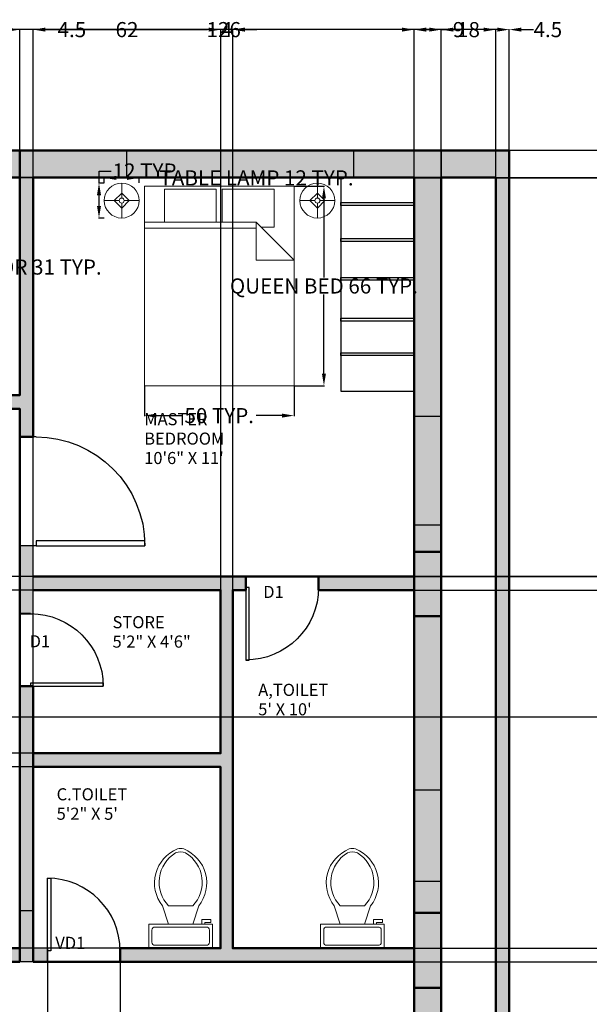
# Model space of a CAD drawing. Units: inches. Extents: x -12 to 887, y 330 to 874.
# Tile 4 of 9: x 253 to 442, y 548 to 874. Entities that reach past the tile are written whole.
import ezdxf

# ---------------------------------------------------------------- set-up
doc = ezdxf.new("R2010")
doc.units = ezdxf.units.IN
doc.header["$MEASUREMENT"] = 0
for name, color, linetype, lineweight in [('A-ANNO-DIMS', 2, 'Continuous', 18), ('A-ANNO-TEXT', 3, 'Continuous', 18), ('A-AREA-IDEN', 7, 'Continuous', 18), ('A-DOOR', 4, 'Continuous', 25), ('A-FLOR-FIXT', 8, 'Continuous', 18), ('A-FLOR-STRS', 3, 'Continuous', 25), ('A-FURN', 9, 'Continuous', 18), ('A-GLAZ', 4, 'Continuous', 25), ('A-WALL', 7, 'Continuous', 50), ('A-WALL-PATT', 5, 'Continuous', 13)]:
    doc.layers.add(name, color=color, linetype=linetype, lineweight=lineweight)
doc.styles.get("Standard").update_dxf_attribs({"font": 'arial.ttf'})
doc.dimstyles.get("Standard").update_dxf_attribs({"dimtxt": 5, "dimasz": 4, "dimexe": 0.18, "dimexo": 0.0625, "dimgap": 0.09, "dimtad": 0, "dimtih": 1, "dimtoh": 1, "dimdec": 1, "dimzin": 0, "dimdsep": 46, "dimlunit": 4, "dimtxsty": 'Standard', "dimcen": 0.09, "dimadec": 0, "dimazin": 0, "dimtfac": 1, "dimtdec": 1, "dimtofl": 0, "dimtmove": 0, "dimatfit": 3, "dimfxl": 1, "dimtolj": 1, "dimtzin": 0, "dimarcsym": 0})

# ---------------------------------------------------------------- blocks, each defined once
blk = doc.blocks.new('*U5')
for p, q in [((0, 0), (0, -6)), ((40, 0), (40, -6))]:
    blk.add_line(p, q)
blk.add_lwpolyline([(0, 0), (0, 40), (1.75, 40), (1.75, 0)], close=True)
blk.add_arc((0, 0), 40, 0, 90)
blk = doc.blocks.new('Bed - Queen')
for p, q in [((0, -80.00003), (0, 0)), ((0, 0), (59.99999, 0)), ((59.99999, 0), (59.99999, -80.00003)), ((7.99999, -1.2), (28.79998, -1.2)), ((7.99999, -14.4), (7.99999, -1.2)), ((28.79998, -1.2), (28.79998, -14.4)), ((31.19999, -1.2), (51.99999, -1.2)), ((31.19999, -14.4), (31.19999, -1.2)), ((51.99999, -1.2), (51.99999, -16.4)), ((0, -14.4), (44.8, -14.4)), ((59.99999, -29.6), (44.8, -14.4)), ((44.8, -14.4), (44.8, -29.6)), ((44.8, -16.8), (0, -16.8)), ((51.99999, -16.4), (46.79936, -16.4)), ((44.8, -29.6), (59.99999, -29.6)), ((59.99999, -80.00003), (0, -80.00003))]:
    blk.add_line(p, q)
blk = doc.blocks.new('Lamp - Table')
for p, q in [((0, 7), (0, 1)), ((-1, 0), (-7, 0)), ((0, 3), (-3, 0)), ((-3, 0), (0, -3)), ((3, 0), (0, 3)), ((0, -3), (3, 0)), ((1, 0), (7, 0)), ((0, -1), (0, -7))]:
    blk.add_line(p, q)
for radius in [7, 1]:
    blk.add_circle((0, 0), radius)
blk = doc.blocks.new('*U12')
for p, q in [((241.3, -152.4), (241.3, -50.8)), ((-254, -215.9), (-203.2, -215.9)), ((-254, -241.3), (-254, -215.9)), ((-177.8, -241.3), (-254, -241.3)), ((-203.2, -215.9), (-203.2, -203.2)), ((-177.8, -203.2), (-177.8, -241.3)), ((-101.6, -203.2), (-152.4, -355.6)), ((101.6, -203.2), (152.4, -355.6)), ((101.6, -355.6), (-101.6, -355.6))]:
    blk.add_line(p, q)
blk.add_lwpolyline([(266.7, -203.2), (266.7, 0), (-266.7, 0), (-266.7, -203.2)], close=True)
for points in [[(-241.3, -50.8), (-241.3, -152.4)], [(215.9, -25.4), (-215.9, -25.4)], [(-215.9, -177.8), (215.9, -177.8)]]:
    blk.add_lwpolyline(points)
for centre, radius, start, end in [((-219.1, -47.6), 22.5, 81.8699, 188.1301), ((219.1, -47.6), 22.5, 351.8699, 98.1301), ((-219.1, -155.6), 22.5, 171.8699, 278.1301), ((219.1, -155.6), 22.5, 261.8699, 8.1301), ((89.4, -548.1), 309.1, 141.46911, 247.97143), ((106.7, -554.2), 287.8, 136.36773, 238.94682), ((-89.4, -548.1), 309.1, 292.02843, 38.53071), ((-106.7, -554.2), 287.8, 301.05301, 43.63209), ((0, -708.1), 101.6, 245.73182, 294.26817), ((0, -736.6), 101.6, 254.86053, 285.13947)]:
    blk.add_arc(centre, radius, start, end)
blk = doc.blocks.new('*D16')
at = {"layer": 'A-ANNO-DIMS', "color": 0, "lineweight": -2, "transparency": 16777216}
for p, q in [((281.4, 819.92), (281.4, 821.77)), ((285.4, 821.59), (288.96, 821.59)), ((292.96, 819.92), (292.96, 821.77)), ((292.96, 821.59), (296.96, 821.59))]:
    blk.add_line(p, q, dxfattribs=at)
at = {"layer": 'A-ANNO-DIMS', "color": 0, "transparency": 16777216}
for points in [[(285.4, 822.26), (285.4, 820.92), (281.4, 821.59)], [(288.96, 822.26), (288.96, 820.92), (292.96, 821.59)]]:
    blk.add_solid(points, dxfattribs=at)
at = {"layer": 'Defpoints', "color": 0, "transparency": 16777216}
for p in [(292.96, 821.59), (281.4, 819.86), (292.96, 819.86)]:
    blk.add_point(p, dxfattribs=at)
at = {"layer": 'A-ANNO-DIMS', "color": 0, "transparency": 16777216, "insert": (331.79, 821.59), "char_height": 5, "attachment_point": 5}
blk.add_mtext('\\A1;TABLE LAMP 12 TYP.', dxfattribs=at)
blk = doc.blocks.new('*D17')
at = {"layer": 'A-ANNO-DIMS', "color": 0, "lineweight": -2, "transparency": 16777216}
for p, q in [((279.67, 819.86), (279.67, 823.86)), ((279.67, 823.86), (283.67, 823.86)), ((281.34, 819.86), (279.49, 819.86)), ((279.67, 812.3), (279.67, 815.86)), ((281.34, 808.3), (279.49, 808.3))]:
    blk.add_line(p, q, dxfattribs=at)
at = {"layer": 'A-ANNO-DIMS', "color": 0, "transparency": 16777216}
for points in [[(279, 815.86), (280.34, 815.86), (279.67, 819.86)], [(279, 812.3), (280.34, 812.3), (279.67, 808.3)]]:
    blk.add_solid(points, dxfattribs=at)
at = {"layer": 'Defpoints', "color": 0, "transparency": 16777216}
for p in [(279.67, 819.86), (281.4, 819.86), (281.4, 808.3)]:
    blk.add_point(p, dxfattribs=at)
at = {"layer": 'A-ANNO-DIMS', "color": 0, "transparency": 16777216, "insert": (295.69, 823.86), "char_height": 5, "attachment_point": 5}
blk.add_mtext('\\A1;12 TYP.', dxfattribs=at)
blk = doc.blocks.new('*D20')
at = {"layer": 'A-ANNO-DIMS', "color": 0, "lineweight": -2, "transparency": 16777216}
for p, q in [((344.26, 818.83), (354.28, 818.83)), ((354.1, 814.83), (354.1, 788.65)), ((354.1, 756.81), (354.1, 782.99)), ((344.26, 752.81), (354.28, 752.81))]:
    blk.add_line(p, q, dxfattribs=at)
at = {"layer": 'A-ANNO-DIMS', "color": 0, "transparency": 16777216}
for points in [[(353.44, 814.83), (354.77, 814.83), (354.1, 818.83)], [(353.44, 756.81), (354.77, 756.81), (354.1, 752.81)]]:
    blk.add_solid(points, dxfattribs=at)
at = {"layer": 'Defpoints', "color": 0, "transparency": 16777216}
for p in [(344.2, 818.83), (354.1, 818.83), (344.2, 752.81)]:
    blk.add_point(p, dxfattribs=at)
at = {"layer": 'A-ANNO-DIMS', "color": 0, "transparency": 16777216, "insert": (354.1, 785.82), "char_height": 5, "attachment_point": 5}
blk.add_mtext('\\A1;QUEEN BED 66 TYP.', dxfattribs=at)
blk = doc.blocks.new('*D21')
at = {"layer": 'A-ANNO-DIMS', "color": 0, "lineweight": -2, "transparency": 16777216}
for p, q in [((294.69, 752.75), (294.69, 742.73)), ((344.2, 752.75), (344.2, 742.73)), ((298.69, 742.91), (307.19, 742.91)), ((340.2, 742.91), (331.7, 742.91))]:
    blk.add_line(p, q, dxfattribs=at)
at = {"layer": 'A-ANNO-DIMS', "color": 0, "transparency": 16777216}
for points in [[(298.69, 743.58), (298.69, 742.24), (294.69, 742.91)], [(340.2, 743.58), (340.2, 742.24), (344.2, 742.91)]]:
    blk.add_solid(points, dxfattribs=at)
at = {"layer": 'Defpoints', "color": 0, "transparency": 16777216}
for p in [(294.69, 752.81), (344.2, 752.81), (344.2, 742.91)]:
    blk.add_point(p, dxfattribs=at)
at = {"layer": 'A-ANNO-DIMS', "color": 0, "transparency": 16777216, "insert": (319.44, 742.91), "char_height": 5, "attachment_point": 5}
blk.add_mtext('\\A1;50 TYP.', dxfattribs=at)
blk = doc.blocks.new('*D28')
at = {"layer": 'A-ANNO-DIMS', "color": 0, "lineweight": -2, "transparency": 16777216}
for p, q in [((167.93, 796.66), (167.93, 791.9)), ((198.86, 796.66), (198.86, 791.9)), ((171.93, 792.08), (194.86, 792.08)), ((198.86, 792.08), (202.86, 792.08))]:
    blk.add_line(p, q, dxfattribs=at)
at = {"layer": 'A-ANNO-DIMS', "color": 0, "transparency": 16777216}
for points in [[(171.93, 792.75), (171.93, 791.42), (167.93, 792.08)], [(194.86, 792.75), (194.86, 791.42), (198.86, 792.08)]]:
    blk.add_solid(points, dxfattribs=at)
at = {"layer": 'Defpoints', "color": 0, "transparency": 16777216}
for p in [(167.93, 796.72), (198.86, 796.72), (198.86, 792.08)]:
    blk.add_point(p, dxfattribs=at)
at = {"layer": 'A-ANNO-DIMS', "color": 0, "transparency": 16777216, "insert": (243.71, 792.08), "char_height": 5, "attachment_point": 5}
blk.add_mtext('\\A1;REFRIGERATOR 31 TYP.', dxfattribs=at)
blk = doc.blocks.new('*D38')
at = {"layer": 'A-ANNO-DIMS', "color": 0, "lineweight": -2, "transparency": 16777216}
for p, q in [((41.93, 830.72), (41.93, 870.84)), ((45.93, 870.66), (220.13, 870.66)), ((411.43, 870.66), (237.22, 870.66)), ((415.43, 830.72), (415.43, 870.84))]:
    blk.add_line(p, q, dxfattribs=at)
at = {"layer": 'A-ANNO-DIMS', "color": 0, "transparency": 16777216}
for points in [[(45.93, 871.33), (45.93, 869.99), (41.93, 870.66)], [(411.43, 871.33), (411.43, 869.99), (415.43, 870.66)]]:
    blk.add_solid(points, dxfattribs=at)
at = {"layer": 'Defpoints', "color": 0, "transparency": 16777216}
for p in [(415.43, 870.66), (41.93, 830.66), (415.43, 830.66)]:
    blk.add_point(p, dxfattribs=at)
at = {"layer": 'A-ANNO-DIMS', "color": 0, "transparency": 16777216, "insert": (228.68, 870.66), "char_height": 5, "attachment_point": 5}
blk.add_mtext('\\A1;373.5', dxfattribs=at)
blk = doc.blocks.new('*D45')
at = {"layer": 'A-ANNO-DIMS', "color": 0, "lineweight": -2, "transparency": 16777216}
for p, q in [((249.43, 870.66), (245.43, 870.66)), ((253.43, 821.72), (253.43, 870.84)), ((257.93, 821.72), (257.93, 870.84)), ((261.93, 870.66), (265.93, 870.66))]:
    blk.add_line(p, q, dxfattribs=at)
at = {"layer": 'A-ANNO-DIMS', "color": 0, "transparency": 16777216}
for points in [[(249.43, 871.33), (249.43, 869.99), (253.43, 870.66)], [(261.93, 871.33), (261.93, 869.99), (257.93, 870.66)]]:
    blk.add_solid(points, dxfattribs=at)
at = {"layer": 'Defpoints', "color": 0, "transparency": 16777216}
for p in [(257.93, 870.66), (253.43, 821.66), (257.93, 821.66)]:
    blk.add_point(p, dxfattribs=at)
at = {"layer": 'A-ANNO-DIMS', "color": 0, "transparency": 16777216, "insert": (270.69, 870.66), "char_height": 5, "attachment_point": 5}
blk.add_mtext('\\A1;4.5', dxfattribs=at)
blk = doc.blocks.new('*D46')
at = {"layer": 'A-ANNO-DIMS', "color": 0, "lineweight": -2, "transparency": 16777216}
for p, q in [((257.93, 821.72), (257.93, 870.84)), ((261.93, 870.66), (315.55, 870.66)), ((379.93, 870.66), (326.3, 870.66)), ((383.93, 821.72), (383.93, 870.84))]:
    blk.add_line(p, q, dxfattribs=at)
at = {"layer": 'A-ANNO-DIMS', "color": 0, "transparency": 16777216}
for points in [[(261.93, 871.33), (261.93, 869.99), (257.93, 870.66)], [(379.93, 871.33), (379.93, 869.99), (383.93, 870.66)]]:
    blk.add_solid(points, dxfattribs=at)
at = {"layer": 'Defpoints', "color": 0, "transparency": 16777216}
for p in [(383.93, 870.66), (257.93, 821.66), (383.93, 821.66)]:
    blk.add_point(p, dxfattribs=at)
at = {"layer": 'A-ANNO-DIMS', "color": 0, "transparency": 16777216, "insert": (320.93, 870.66), "char_height": 5, "attachment_point": 5}
blk.add_mtext('\\A1;126', dxfattribs=at)
blk = doc.blocks.new('*D47')
at = {"layer": 'A-ANNO-DIMS', "color": 0, "lineweight": -2, "transparency": 16777216}
for p, q in [((383.93, 821.72), (383.93, 870.84)), ((387.93, 870.66), (388.93, 870.66)), ((392.93, 821.72), (392.93, 870.84)), ((392.93, 870.66), (396.93, 870.66))]:
    blk.add_line(p, q, dxfattribs=at)
at = {"layer": 'A-ANNO-DIMS', "color": 0, "transparency": 16777216}
for points in [[(387.93, 871.33), (387.93, 869.99), (383.93, 870.66)], [(388.93, 871.33), (388.93, 869.99), (392.93, 870.66)]]:
    blk.add_solid(points, dxfattribs=at)
at = {"layer": 'Defpoints', "color": 0, "transparency": 16777216}
for p in [(392.93, 870.66), (383.93, 821.66), (392.93, 821.66)]:
    blk.add_point(p, dxfattribs=at)
at = {"layer": 'A-ANNO-DIMS', "color": 0, "transparency": 16777216, "insert": (398.66, 870.66), "char_height": 5, "attachment_point": 5}
blk.add_mtext('\\A1;9', dxfattribs=at)
blk = doc.blocks.new('*D48')
at = {"layer": 'A-ANNO-DIMS', "color": 0, "lineweight": -2, "transparency": 16777216}
for p, q in [((392.93, 821.72), (392.93, 870.84)), ((396.93, 870.66), (398.49, 870.66)), ((406.93, 870.66), (405.37, 870.66)), ((410.93, 821.72), (410.93, 870.84))]:
    blk.add_line(p, q, dxfattribs=at)
at = {"layer": 'A-ANNO-DIMS', "color": 0, "transparency": 16777216}
for points in [[(396.93, 871.33), (396.93, 869.99), (392.93, 870.66)], [(406.93, 871.33), (406.93, 869.99), (410.93, 870.66)]]:
    blk.add_solid(points, dxfattribs=at)
at = {"layer": 'Defpoints', "color": 0, "transparency": 16777216}
for p in [(410.93, 870.66), (392.93, 821.66), (410.93, 821.66)]:
    blk.add_point(p, dxfattribs=at)
at = {"layer": 'A-ANNO-DIMS', "color": 0, "transparency": 16777216, "insert": (401.93, 870.66), "char_height": 5, "attachment_point": 5}
blk.add_mtext('\\A1;18', dxfattribs=at)
blk = doc.blocks.new('*D49')
at = {"layer": 'A-ANNO-DIMS', "color": 0, "lineweight": -2, "transparency": 16777216}
for p, q in [((406.93, 870.66), (402.93, 870.66)), ((410.93, 821.72), (410.93, 870.84)), ((415.43, 830.72), (415.43, 870.84)), ((419.43, 870.66), (423.43, 870.66))]:
    blk.add_line(p, q, dxfattribs=at)
at = {"layer": 'A-ANNO-DIMS', "color": 0, "transparency": 16777216}
for points in [[(406.93, 871.33), (406.93, 869.99), (410.93, 870.66)], [(419.43, 871.33), (419.43, 869.99), (415.43, 870.66)]]:
    blk.add_solid(points, dxfattribs=at)
at = {"layer": 'Defpoints', "color": 0, "transparency": 16777216}
for p in [(415.43, 870.66), (415.43, 830.66), (410.93, 821.66)]:
    blk.add_point(p, dxfattribs=at)
at = {"layer": 'A-ANNO-DIMS', "color": 0, "transparency": 16777216, "insert": (428.19, 870.66), "char_height": 5, "attachment_point": 5}
blk.add_mtext('\\A1;4.5', dxfattribs=at)
blk = doc.blocks.new('*D62')
at = {"layer": 'A-ANNO-DIMS', "color": 0, "lineweight": -2, "transparency": 16777216}
for p, q in [((383.99, 562.16), (873.75, 562.16)), ((873.57, 558.16), (873.57, 510.8)), ((873.57, 458.16), (873.57, 505.52)), ((383.99, 454.16), (873.75, 454.16))]:
    blk.add_line(p, q, dxfattribs=at)
at = {"layer": 'A-ANNO-DIMS', "color": 0, "transparency": 16777216}
for points in [[(872.9, 558.16), (874.24, 558.16), (873.57, 562.16)], [(872.9, 458.16), (874.24, 458.16), (873.57, 454.16)]]:
    blk.add_solid(points, dxfattribs=at)
at = {"layer": 'Defpoints', "color": 0, "transparency": 16777216}
for p in [(383.93, 562.16), (873.57, 562.16), (383.93, 454.16)]:
    blk.add_point(p, dxfattribs=at)
at = {"layer": 'A-ANNO-DIMS', "color": 0, "transparency": 16777216, "insert": (873.57, 508.16), "char_height": 5, "attachment_point": 5}
blk.add_mtext('\\A1;108', dxfattribs=at)
blk = doc.blocks.new('*D63')
at = {"layer": 'A-ANNO-DIMS', "color": 0, "lineweight": -2, "transparency": 16777216}
for p, q in [((873.57, 570.66), (873.57, 574.66)), ((873.57, 574.66), (877.57, 574.66)), ((383.99, 566.66), (873.75, 566.66)), ((383.99, 562.16), (873.75, 562.16)), ((873.57, 558.16), (873.57, 554.16))]:
    blk.add_line(p, q, dxfattribs=at)
at = {"layer": 'A-ANNO-DIMS', "color": 0, "transparency": 16777216}
for points in [[(872.9, 570.66), (874.24, 570.66), (873.57, 566.66)], [(872.9, 558.16), (874.24, 558.16), (873.57, 562.16)]]:
    blk.add_solid(points, dxfattribs=at)
at = {"layer": 'Defpoints', "color": 0, "transparency": 16777216}
for p in [(383.93, 566.66), (873.57, 566.66), (383.93, 562.16)]:
    blk.add_point(p, dxfattribs=at)
at = {"layer": 'A-ANNO-DIMS', "color": 0, "transparency": 16777216, "insert": (882.33, 574.66), "char_height": 5, "attachment_point": 5}
blk.add_mtext('\\A1;4.5', dxfattribs=at)
blk = doc.blocks.new('*D64')
at = {"layer": 'A-ANNO-DIMS', "color": 0, "lineweight": -2, "transparency": 16777216}
for p, q in [((383.99, 685.16), (873.75, 685.16)), ((873.57, 681.16), (873.57, 628.55)), ((873.57, 570.66), (873.57, 623.27)), ((383.99, 566.66), (873.75, 566.66))]:
    blk.add_line(p, q, dxfattribs=at)
at = {"layer": 'A-ANNO-DIMS', "color": 0, "transparency": 16777216}
for points in [[(872.9, 681.16), (874.24, 681.16), (873.57, 685.16)], [(872.9, 570.66), (874.24, 570.66), (873.57, 566.66)]]:
    blk.add_solid(points, dxfattribs=at)
at = {"layer": 'Defpoints', "color": 0, "transparency": 16777216}
for p in [(383.93, 685.16), (873.57, 685.16), (383.93, 566.66)]:
    blk.add_point(p, dxfattribs=at)
at = {"layer": 'A-ANNO-DIMS', "color": 0, "transparency": 16777216, "insert": (873.57, 625.91), "char_height": 5, "attachment_point": 5}
blk.add_mtext('\\A1;118.5', dxfattribs=at)
blk = doc.blocks.new('*D65')
at = {"layer": 'A-ANNO-DIMS', "color": 0, "lineweight": -2, "transparency": 16777216}
for p, q in [((873.57, 693.66), (873.57, 697.66)), ((873.57, 697.66), (877.57, 697.66)), ((383.99, 689.66), (873.75, 689.66)), ((383.99, 685.16), (873.75, 685.16)), ((873.57, 681.16), (873.57, 677.16))]:
    blk.add_line(p, q, dxfattribs=at)
at = {"layer": 'A-ANNO-DIMS', "color": 0, "transparency": 16777216}
for points in [[(872.9, 693.66), (874.24, 693.66), (873.57, 689.66)], [(872.9, 681.16), (874.24, 681.16), (873.57, 685.16)]]:
    blk.add_solid(points, dxfattribs=at)
at = {"layer": 'Defpoints', "color": 0, "transparency": 16777216}
for p in [(383.93, 689.66), (873.57, 689.66), (383.93, 685.16)]:
    blk.add_point(p, dxfattribs=at)
at = {"layer": 'A-ANNO-DIMS', "color": 0, "transparency": 16777216, "insert": (882.33, 697.66), "char_height": 5, "attachment_point": 5}
blk.add_mtext('\\A1;4.5', dxfattribs=at)
blk = doc.blocks.new('*D66')
at = {"layer": 'A-ANNO-DIMS', "color": 0, "lineweight": -2, "transparency": 16777216}
for p, q in [((383.99, 821.66), (873.75, 821.66)), ((873.57, 817.66), (873.57, 758.31)), ((873.57, 693.66), (873.57, 753.02)), ((383.99, 689.66), (873.75, 689.66))]:
    blk.add_line(p, q, dxfattribs=at)
at = {"layer": 'A-ANNO-DIMS', "color": 0, "transparency": 16777216}
for points in [[(872.9, 817.66), (874.24, 817.66), (873.57, 821.66)], [(872.9, 693.66), (874.24, 693.66), (873.57, 689.66)]]:
    blk.add_solid(points, dxfattribs=at)
at = {"layer": 'Defpoints', "color": 0, "transparency": 16777216}
for p in [(383.93, 821.66), (873.57, 821.66), (383.93, 689.66)]:
    blk.add_point(p, dxfattribs=at)
at = {"layer": 'A-ANNO-DIMS', "color": 0, "transparency": 16777216, "insert": (873.57, 755.66), "char_height": 5, "attachment_point": 5}
blk.add_mtext('\\A1;132', dxfattribs=at)
blk = doc.blocks.new('*D67')
at = {"layer": 'A-ANNO-DIMS', "color": 0, "lineweight": -2, "transparency": 16777216}
for p, q in [((319.86, 626.66), (1.75, 626.66)), ((1.93, 622.66), (1.93, 599.3)), ((1.93, 570.66), (1.93, 594.02)), ((319.86, 566.66), (1.75, 566.66))]:
    blk.add_line(p, q, dxfattribs=at)
at = {"layer": 'A-ANNO-DIMS', "color": 0, "transparency": 16777216}
for points in [[(1.26, 622.66), (2.59, 622.66), (1.93, 626.66)], [(1.26, 570.66), (2.59, 570.66), (1.93, 566.66)]]:
    blk.add_solid(points, dxfattribs=at)
at = {"layer": 'Defpoints', "color": 0, "transparency": 16777216}
for p in [(1.93, 626.66), (319.93, 626.66), (319.93, 566.66)]:
    blk.add_point(p, dxfattribs=at)
at = {"layer": 'A-ANNO-DIMS', "color": 0, "transparency": 16777216, "insert": (1.93, 596.66), "char_height": 5, "attachment_point": 5}
blk.add_mtext('\\A1;60', dxfattribs=at)
blk = doc.blocks.new('*D68')
at = {"layer": 'A-ANNO-DIMS', "color": 0, "lineweight": -2, "transparency": 16777216}
for p, q in [((1.93, 635.16), (1.93, 639.16)), ((1.93, 639.16), (5.93, 639.16)), ((319.86, 631.16), (1.75, 631.16)), ((319.86, 626.66), (1.75, 626.66)), ((1.93, 622.66), (1.93, 618.66))]:
    blk.add_line(p, q, dxfattribs=at)
at = {"layer": 'A-ANNO-DIMS', "color": 0, "transparency": 16777216}
for points in [[(1.26, 635.16), (2.59, 635.16), (1.93, 631.16)], [(1.26, 622.66), (2.59, 622.66), (1.93, 626.66)]]:
    blk.add_solid(points, dxfattribs=at)
at = {"layer": 'Defpoints', "color": 0, "transparency": 16777216}
for p in [(1.93, 631.16), (319.93, 631.16), (319.93, 626.66)]:
    blk.add_point(p, dxfattribs=at)
at = {"layer": 'A-ANNO-DIMS', "color": 0, "transparency": 16777216, "insert": (10.69, 639.16), "char_height": 5, "attachment_point": 5}
blk.add_mtext('\\A1;4.5', dxfattribs=at)
blk = doc.blocks.new('*D69')
at = {"layer": 'A-ANNO-DIMS', "color": 0, "lineweight": -2, "transparency": 16777216}
for p, q in [((319.86, 685.16), (1.75, 685.16)), ((1.93, 681.16), (1.93, 660.79)), ((1.93, 635.16), (1.93, 655.53)), ((319.86, 631.16), (1.75, 631.16))]:
    blk.add_line(p, q, dxfattribs=at)
at = {"layer": 'A-ANNO-DIMS', "color": 0, "transparency": 16777216}
for points in [[(1.26, 681.16), (2.59, 681.16), (1.93, 685.16)], [(1.26, 635.16), (2.59, 635.16), (1.93, 631.16)]]:
    blk.add_solid(points, dxfattribs=at)
at = {"layer": 'Defpoints', "color": 0, "transparency": 16777216}
for p in [(1.93, 685.16), (319.93, 685.16), (319.93, 631.16)]:
    blk.add_point(p, dxfattribs=at)
at = {"layer": 'A-ANNO-DIMS', "color": 0, "transparency": 16777216, "insert": (1.93, 658.16), "char_height": 5, "attachment_point": 5}
blk.add_mtext('\\A1;54', dxfattribs=at)
blk = doc.blocks.new('*D70')
at = {"layer": 'A-ANNO-DIMS', "color": 0, "lineweight": -2, "transparency": 16777216}
for p, q in [((257.93, 631.22), (257.93, 870.84)), ((261.93, 870.66), (285.27, 870.66)), ((315.93, 870.66), (292.59, 870.66)), ((319.93, 631.22), (319.93, 870.84))]:
    blk.add_line(p, q, dxfattribs=at)
at = {"layer": 'A-ANNO-DIMS', "color": 0, "transparency": 16777216}
for points in [[(261.93, 871.33), (261.93, 869.99), (257.93, 870.66)], [(315.93, 871.33), (315.93, 869.99), (319.93, 870.66)]]:
    blk.add_solid(points, dxfattribs=at)
at = {"layer": 'Defpoints', "color": 0, "transparency": 16777216}
for p in [(319.93, 870.66), (257.93, 631.16), (319.93, 631.16)]:
    blk.add_point(p, dxfattribs=at)
at = {"layer": 'A-ANNO-DIMS', "color": 0, "transparency": 16777216, "insert": (288.93, 870.66), "char_height": 5, "attachment_point": 5}
blk.add_mtext('\\A1;62', dxfattribs=at)
blk = doc.blocks.new('*D71')
at = {"layer": 'A-ANNO-DIMS', "color": 0, "lineweight": -2, "transparency": 16777216}
for p, q in [((315.93, 870.66), (311.93, 870.66)), ((319.93, 685.22), (319.93, 870.84)), ((323.93, 685.22), (323.93, 870.84)), ((327.93, 870.66), (331.93, 870.66))]:
    blk.add_line(p, q, dxfattribs=at)
at = {"layer": 'A-ANNO-DIMS', "color": 0, "transparency": 16777216}
for points in [[(315.93, 871.33), (315.93, 869.99), (319.93, 870.66)], [(327.93, 871.33), (327.93, 869.99), (323.93, 870.66)]]:
    blk.add_solid(points, dxfattribs=at)
at = {"layer": 'Defpoints', "color": 0, "transparency": 16777216}
for p in [(323.93, 870.66), (319.93, 685.16), (323.93, 685.16)]:
    blk.add_point(p, dxfattribs=at)
at = {"layer": 'A-ANNO-DIMS', "color": 0, "transparency": 16777216, "insert": (321.93, 870.66), "char_height": 5, "attachment_point": 5}
blk.add_mtext('\\A1;4', dxfattribs=at)
blk = doc.blocks.new('*D80')
at = {"layer": 'A-ANNO-DIMS', "color": 0, "lineweight": -2, "transparency": 16777216}
for p, q in [((262.63, 566.6), (262.63, 332.98)), ((286.63, 566.6), (286.63, 332.98)), ((266.63, 333.16), (270.92, 333.16)), ((282.63, 333.16), (278.33, 333.16))]:
    blk.add_line(p, q, dxfattribs=at)
at = {"layer": 'A-ANNO-DIMS', "color": 0, "transparency": 16777216}
for points in [[(266.63, 333.83), (266.63, 332.49), (262.63, 333.16)], [(282.63, 333.83), (282.63, 332.49), (286.63, 333.16)]]:
    blk.add_solid(points, dxfattribs=at)
at = {"layer": 'Defpoints', "color": 0, "transparency": 16777216}
for p in [(262.63, 566.66), (286.63, 566.66), (286.63, 333.16)]:
    blk.add_point(p, dxfattribs=at)
at = {"layer": 'A-ANNO-DIMS', "color": 0, "transparency": 16777216, "insert": (274.63, 333.16), "char_height": 5, "attachment_point": 5}
blk.add_mtext('\\A1;24', dxfattribs=at)
blk = doc.blocks.new('*D101')
at = {"layer": 'A-ANNO-DIMS', "color": 0, "lineweight": -2, "transparency": 16777216}
for p, q in [((493.01, 643.16), (1.75, 643.16)), ((1.93, 639.16), (1.93, 551.3)), ((1.93, 458.16), (1.93, 546.02)), ((493.01, 454.16), (1.75, 454.16))]:
    blk.add_line(p, q, dxfattribs=at)
at = {"layer": 'A-ANNO-DIMS', "color": 0, "transparency": 16777216}
for points in [[(1.26, 639.16), (2.59, 639.16), (1.93, 643.16)], [(1.26, 458.16), (2.59, 458.16), (1.93, 454.16)]]:
    blk.add_solid(points, dxfattribs=at)
at = {"layer": 'Defpoints', "color": 0, "transparency": 16777216}
for p in [(1.93, 643.16), (493.07, 643.16), (493.07, 454.16)]:
    blk.add_point(p, dxfattribs=at)
at = {"layer": 'A-ANNO-DIMS', "color": 0, "transparency": 16777216, "insert": (1.93, 548.66), "char_height": 5, "attachment_point": 5}
blk.add_mtext('\\A1;189', dxfattribs=at)
blk = doc.blocks.new('*D102')
at = {"layer": 'A-ANNO-DIMS', "color": 0, "lineweight": -2, "transparency": 16777216}
for p, q in [((493.01, 821.66), (1.75, 821.66)), ((1.93, 817.66), (1.93, 735.05)), ((1.93, 647.16), (1.93, 729.77)), ((493.01, 643.16), (1.75, 643.16))]:
    blk.add_line(p, q, dxfattribs=at)
at = {"layer": 'A-ANNO-DIMS', "color": 0, "transparency": 16777216}
for points in [[(1.26, 817.66), (2.59, 817.66), (1.93, 821.66)], [(1.26, 647.16), (2.59, 647.16), (1.93, 643.16)]]:
    blk.add_solid(points, dxfattribs=at)
at = {"layer": 'Defpoints', "color": 0, "transparency": 16777216}
for p in [(1.93, 821.66), (493.07, 821.66), (493.07, 643.16)]:
    blk.add_point(p, dxfattribs=at)
at = {"layer": 'A-ANNO-DIMS', "color": 0, "transparency": 16777216, "insert": (1.93, 732.41), "char_height": 5, "attachment_point": 5}
blk.add_mtext('\\A1;178.5', dxfattribs=at)
blk = doc.blocks.new('*D103')
at = {"layer": 'A-ANNO-DIMS', "color": 0, "lineweight": -2, "transparency": 16777216}
for p, q in [((1.93, 830.66), (1.93, 834.66)), ((1.93, 834.66), (5.93, 834.66)), ((460.01, 830.66), (1.75, 830.66)), ((1.93, 825.66), (1.93, 826.66)), ((493.01, 821.66), (1.75, 821.66))]:
    blk.add_line(p, q, dxfattribs=at)
at = {"layer": 'A-ANNO-DIMS', "color": 0, "transparency": 16777216}
for points in [[(1.26, 826.66), (2.59, 826.66), (1.93, 830.66)], [(1.26, 825.66), (2.59, 825.66), (1.93, 821.66)]]:
    blk.add_solid(points, dxfattribs=at)
at = {"layer": 'Defpoints', "color": 0, "transparency": 16777216}
for p in [(1.93, 830.66), (460.07, 830.66), (493.07, 821.66)]:
    blk.add_point(p, dxfattribs=at)
at = {"layer": 'A-ANNO-DIMS', "color": 0, "transparency": 16777216, "insert": (7.66, 834.66), "char_height": 5, "attachment_point": 5}
blk.add_mtext('\\A1;9', dxfattribs=at)
blk = doc.blocks.new('*D112')
at = {"layer": 'A-ANNO-DIMS', "color": 0, "lineweight": -2, "transparency": 16777216}
for p, q in [((676.01, 821.66), (1.75, 821.66)), ((1.93, 817.66), (1.93, 758.31)), ((1.93, 693.66), (1.93, 753.02)), ((676.01, 689.66), (1.75, 689.66))]:
    blk.add_line(p, q, dxfattribs=at)
at = {"layer": 'A-ANNO-DIMS', "color": 0, "transparency": 16777216}
for points in [[(1.26, 817.66), (2.59, 817.66), (1.93, 821.66)], [(1.26, 693.66), (2.59, 693.66), (1.93, 689.66)]]:
    blk.add_solid(points, dxfattribs=at)
at = {"layer": 'Defpoints', "color": 0, "transparency": 16777216}
for p in [(1.93, 821.66), (676.07, 821.66), (676.07, 689.66)]:
    blk.add_point(p, dxfattribs=at)
at = {"layer": 'A-ANNO-DIMS', "color": 0, "transparency": 16777216, "insert": (1.93, 755.66), "char_height": 5, "attachment_point": 5}
blk.add_mtext('\\A1;132', dxfattribs=at)

msp = doc.modelspace()

# ---------------------------------------------------------------- hatches: boundary and pattern name
at = {"layer": 'A-WALL-PATT'}
h = msp.add_hatch(color=256, dxfattribs=at)
h.dxf.hatch_style = 1
h.paths.add_polyline_path([(253.4263, 830.6611), (94.575, 830.6611), (94.575, 821.6611), (198.9263, 821.6611), (198.9263, 783.3094), (203.4263, 783.3094), (203.4263, 821.6611), (253.4263, 821.6611)], flags=17)
h.paths.add_polyline_path([(415.4263, 830.6611), (392.9263, 830.6611), (392.9263, 821.6611), (410.9263, 821.6611), (410.9263, 701.6611), (410.9263, 382.1611), (392.9263, 382.1611), (392.9263, 450.1611), (383.9263, 450.1611), (383.9263, 382.1611), (253.4263, 382.1611), (46.4263, 382.1611), (46.4263, 821.6611), (67.3199, 821.6611), (67.3199, 830.6611), (41.9263, 830.6611), (41.9263, 373.1611), (253.4263, 373.1611), (415.4263, 373.1611)])
h.paths.add_polyline_path([(364.023, 830.6611), (288.8031, 830.6611), (288.8031, 821.6611), (364.023, 821.6611)], flags=17)
h.paths.add_polyline_path([(257.9263, 821.6611), (253.4263, 821.6611), (253.4263, 749.6611), (203.4263, 749.6611), (203.4263, 759.3094), (198.9263, 759.3094), (198.9263, 745.1611), (253.4263, 745.1611), (253.4263, 735.8547), (257.9263, 735.8547)], flags=17)
h.paths.add_polyline_path([(257.9263, 653.338), (257.0311, 653.338), (253.4263, 653.338), (253.4263, 579.1607), (257.9263, 579.1607)], flags=17)
h.paths.add_polyline_path([(323.9263, 685.1611), (328.2749, 685.1611), (328.2749, 689.6611), (257.9263, 689.6611), (257.9263, 685.1611), (319.9263, 685.1611), (319.9263, 631.1611), (257.9263, 631.1611), (257.9263, 626.6611), (319.9263, 626.6611), (319.9263, 566.6611), (286.6409, 566.6611, -0.00931598), (286.6576, 565.7658), (286.6576, 562.1611), (383.9263, 562.1611), (383.9263, 566.6611), (323.9263, 566.6611)], flags=17)
h.paths.add_polyline_path([(142.5107, 566.6611), (135.5357, 566.6611), (135.5357, 562.1611), (142.5107, 562.1611)], flags=17)
h.paths.add_polyline_path([(253.4263, 566.6611), (229.0035, 566.6611), (229.0035, 562.1611), (253.4263, 562.1611)], flags=17)
h.paths.add_polyline_path([(262.6261, 566.6611), (257.9263, 566.6611), (257.9263, 562.1611), (262.6261, 562.1611)], flags=17)
h.paths.add_polyline_path([(392.9263, 553.5254), (383.9263, 553.5254), (383.9263, 454.1611), (392.9263, 454.1611)], flags=17)
h.paths.add_polyline_path([(353.8031, 418.1611), (247.9263, 418.1611), (247.9263, 414.1611), (353.8031, 414.1611)], flags=17)
h.paths.add_polyline_path([(374.959, 454.1611), (272.0195, 454.1611), (272.0195, 450.1611), (374.959, 450.1611)], flags=17)
h.paths.add_polyline_path([(254.2006, 454.1611), (247.9263, 454.1611), (247.9263, 450.1611), (254.2006, 450.1611)], flags=17)
h = msp.add_hatch(color=256, dxfattribs=at)
h.dxf.hatch_style = 1
h.paths.add_polyline_path([(94.575, 830.6611), (67.3199, 830.6611), (67.3199, 821.6611), (70.4263, 821.6611), (79.4263, 821.6611), (94.575, 821.6611)])
h.paths.add_polyline_path([(288.8031, 830.6611), (257.9263, 830.6611), (253.4263, 830.6611), (253.4263, 821.6611), (288.8031, 821.6611)])
h.paths.add_polyline_path([(74.9263, 696.9265), (70.4263, 696.9265), (70.4263, 678.4656), (74.9263, 678.4656)])
h.paths.add_polyline_path([(74.9263, 584.8756), (70.4263, 584.8756), (70.4263, 562.1611), (74.9263, 562.1611)])
h.paths.add_polyline_path([(135.5357, 566.6611), (122.6994, 566.6611), (122.6994, 562.1611), (135.5357, 562.1611)])
h.paths.add_polyline_path([(257.9263, 579.1607), (253.4263, 579.1607), (253.4263, 562.1611), (257.9263, 562.1611)])
h.paths.add_polyline_path([(272.0195, 454.1611), (254.2006, 454.1611), (254.2006, 450.1611), (272.0195, 450.1611)])
h.paths.add_polyline_path([(392.9263, 454.1611), (374.959, 454.1611), (374.959, 450.1611), (383.9263, 450.1611), (392.9263, 450.1611)])
h.paths.add_polyline_path([(493.0683, 466.4171), (488.5683, 466.4171), (488.5683, 450.1611), (493.0683, 450.1611)])
h.paths.add_polyline_path([(568.6302, 454.1611), (555.938, 454.1611), (555.938, 450.1611), (568.6302, 450.1611)])
h.paths.add_polyline_path([(493.0683, 594.9471), (488.5683, 594.9471), (488.5683, 569.5862), (493.0683, 569.5862)])
h.paths.add_polyline_path([(690.1615, 454.1611), (672.3426, 454.1611), (672.3426, 450.1611), (690.1615, 450.1611)])
h.paths.add_polyline_path([(811.0683, 454.1611), (793.101, 454.1611), (793.101, 450.1611), (802.0683, 450.1611), (811.0683, 450.1611)])
h.paths.add_polyline_path([(811.0683, 578.3606), (802.0683, 578.3606), (802.0683, 566.6611), (802.0683, 553.5254), (811.0683, 553.5254)])
h.paths.add_polyline_path([(811.0683, 701.6611), (802.0683, 701.6611), (802.0683, 689.9616), (802.0683, 676.8259), (811.0683, 676.8259)])
h.paths.add_polyline_path([(811.0683, 830.6611), (782.165, 830.6611), (782.165, 821.6611), (802.0683, 821.6611), (811.0683, 821.6611)])
h.paths.add_polyline_path([(706.9451, 830.6611), (671.5683, 830.6611), (671.5683, 821.6611), (706.9451, 821.6611)])
h.paths.add_polyline_path([(512.717, 830.6611), (485.4619, 830.6611), (485.4619, 821.6611), (488.5683, 821.6611), (512.717, 821.6611)])
h.paths.add_polyline_path([(392.9263, 697.8668), (383.9263, 697.8668), (383.9263, 689.6611), (383.9263, 676.5034), (392.9263, 676.5034)])
h.paths.add_polyline_path([(392.9263, 830.6611), (364.023, 830.6611), (364.023, 821.7357), (392.9263, 821.7357)])
h.paths.add_polyline_path([(392.9263, 619.0434), (383.9263, 619.0434), (383.9263, 588.7499), (392.9263, 588.7499)])
h.paths.add_polyline_path([(392.9263, 578.3606), (383.9263, 578.3606), (383.9263, 566.6611), (383.9263, 553.5254), (392.9263, 553.5254)])
h.paths.add_polyline_path([(257.9263, 699.8547), (253.4263, 699.8547), (253.4263, 697.1611), (253.4263, 677.338), (257.9263, 677.338)])
h.paths.add_polyline_path([(493.0683, 714.3785), (488.5683, 714.3785), (488.5683, 689.6611), (493.0683, 689.6611)])
h.paths.add_polyline_path([(74.9263, 491.4191), (70.4263, 491.4191), (70.4263, 480.7097), (74.9263, 480.7097)])
h = msp.add_hatch(color=256, dxfattribs=at)
h.dxf.hatch_style = 1
h.paths.add_polyline_path([(86.6469, 566.6611), (74.9263, 566.6611), (74.9263, 562.1611), (86.6469, 562.1611)])
h.paths.add_polyline_path([(74.9263, 599.271), (70.4263, 599.271), (70.4263, 584.8756), (74.9263, 584.8756)])
h.paths.add_polyline_path([(74.9263, 678.4656), (70.4263, 678.4656), (70.4263, 671.2153), (74.9263, 671.2153)])
h.paths.add_polyline_path([(74.9263, 709.2627), (70.4263, 709.2627), (70.4263, 696.9265), (74.9263, 696.9265)])
h.paths.add_polyline_path([(74.9263, 821.6611), (70.4263, 821.6611), (70.4263, 749.8953), (74.9263, 749.8953)])
h.paths.add_polyline_path([(383.9263, 689.6611), (352.3064, 689.6611), (352.3064, 686.0564, -0.00931598), (352.2897, 685.1611), (383.9263, 685.1611)])
h.paths.add_polyline_path([(392.9263, 706.6608), (383.9263, 706.6608), (383.9263, 701.6611), (383.9263, 697.8668), (392.9263, 697.8668)])
h.paths.add_polyline_path([(392.9263, 821.7357), (383.9263, 821.7357), (383.9263, 751.0224), (383.9263, 742.7561), (392.9263, 742.7561)])
h.paths.add_polyline_path([(392.9263, 676.5034), (383.9263, 676.5034), (383.9263, 619.0434), (392.9263, 619.0434)])
h.paths.add_polyline_path([(392.9263, 588.7499), (383.9263, 588.7499), (383.9263, 578.3606), (392.9263, 578.3606)])
h = msp.add_hatch(color=256, dxfattribs=at)
h.dxf.hatch_style = 1
h.paths.add_polyline_path([(74.9263, 749.8953), (70.4263, 749.8953), (70.4263, 709.2627), (74.9263, 709.2627)])
h.paths.add_polyline_path([(74.9263, 671.2153), (70.4263, 671.2153), (70.4263, 599.271), (74.9263, 599.271)])
h.paths.add_polyline_path([(229.0035, 566.6611), (142.5107, 566.6611), (142.5107, 562.1611), (229.0035, 562.1611)])
h.paths.add_polyline_path([(392.9263, 742.7561), (383.9263, 742.7561), (383.9263, 706.6608), (392.9263, 706.6608)])
h.paths.add_polyline_path([(656.7304, 454.1611), (582.6585, 454.1611), (582.6585, 450.1611), (656.7304, 450.1611)])
h.paths.add_polyline_path([(493.0683, 557.2595), (488.5683, 557.2595), (488.5683, 492.3446), (493.0683, 492.3446)])
h.paths.add_polyline_path([(493.0683, 781.3634), (488.5683, 781.3634), (488.5683, 728.8273), (493.0683, 728.8273)])
h.paths.add_polyline_path([(811.0683, 756.0738), (802.0683, 756.0738), (802.0683, 707.8935), (811.0683, 707.8935)])

# ---------------------------------------------------------------- linework, layer by layer
at = {"layer": 'A-FLOR-STRS'}
for points in [[(383.9263, 821.6611), (359.6676, 821.6611), (359.6676, 751.0224), (383.9263, 751.0224)], [(359.6676, 813.3906), (383.9263, 813.3906), (383.9263, 812.4725), (359.6676, 812.4725)], [(359.6676, 801.477), (383.9263, 801.477), (383.9263, 800.5589), (359.6676, 800.5589)], [(359.6676, 788.6179), (383.9263, 788.6179), (383.9263, 787.6997), (359.6676, 787.6997)], [(359.6676, 775.1314), (383.9263, 775.1314), (383.9263, 774.2133), (359.6676, 774.2133)], [(359.6676, 763.6836), (383.9263, 763.6836), (383.9263, 762.7655), (359.6676, 762.7655)]]:
    msp.add_lwpolyline(points, close=True, dxfattribs=at)
at = {"layer": 'A-GLAZ'}
for points in [[(253.4263, 830.6611), (288.8031, 830.6611), (288.8031, 821.6611), (253.4263, 821.6611)], [(392.9263, 821.7357), (364.023, 821.7357), (364.023, 830.6611), (392.9263, 830.6611)], [(392.9263, 706.6608), (383.9263, 706.6608), (383.9263, 742.7561), (392.9263, 742.7561)], [(383.9263, 619.0434), (392.9263, 619.0434), (392.9263, 588.7499), (383.9263, 588.7499)], [(257.9263, 562.1611), (253.4263, 562.1611), (253.4263, 579.1607), (257.9263, 579.1607)]]:
    msp.add_lwpolyline(points, close=True, dxfattribs=at)
for points in [[(253.4263, 677.338), (257.9263, 677.338), (257.9263, 699.8547), (253.4263, 699.8547)], [(262.6261, 562.1611), (262.6261, 566.6611), (257.9263, 566.6611)]]:
    msp.add_lwpolyline(points, dxfattribs=at)
at = {"layer": 'A-WALL'}
for p, q in [((257.9263, 653.338), (253.4263, 653.338)), ((257.9263, 653.338), (257.9263, 562.1611)), ((122.6994, 566.6611), (253.4263, 566.6611)), ((257.9263, 562.1611), (383.9263, 562.1611)), ((383.9263, 562.1611), (383.9263, 454.1611))]:
    msp.add_line(p, q, dxfattribs=at)
for points in [[(41.9263, 830.6611), (253.4263, 830.6611), (257.9263, 830.6611), (415.4263, 830.6611), (415.4263, 373.1611), (253.4263, 373.1611), (41.9263, 373.1611)], [(410.9263, 821.6611), (392.9263, 821.6611), (392.9263, 382.1611), (410.9263, 382.1611), (410.9263, 701.6611)]]:
    msp.add_lwpolyline(points, close=True, dxfattribs=at)
for points in [[(198.9263, 759.3094), (203.4263, 759.3094), (203.4263, 749.6611), (253.4263, 749.6611), (253.4263, 830.6611)], [(253.4263, 821.6611), (203.4263, 821.6611), (203.4263, 783.3094), (198.9263, 783.3094)], [(253.4263, 735.8547), (257.9263, 735.8547), (257.9263, 821.6611), (383.9263, 821.6611), (383.9263, 701.6611), (383.9263, 689.6611), (383.9263, 697.8668), (392.9263, 697.8668), (392.9263, 676.5034), (383.9263, 676.5034), (383.9263, 689.6611), (257.9263, 689.6611)], [(86.6469, 562.1611), (86.6469, 566.6611), (74.9263, 566.6611), (74.9263, 685.1611), (198.9263, 685.1611), (198.9263, 745.1611), (253.4263, 745.1611), (253.4263, 697.1611), (253.4263, 562.1611), (122.6469, 562.1611)], [(383.9263, 626.6611), (383.9263, 566.6611), (383.9263, 578.3606), (392.9263, 578.3606), (392.9263, 553.5254), (383.9263, 553.5254), (383.9263, 566.6611), (323.9263, 566.6611), (323.9263, 685.1611), (328.2749, 685.1611), (328.2749, 689.6611)], [(383.9263, 577.1611), (383.9263, 685.1611), (352.2749, 685.1611), (352.2749, 689.6611)], [(257.9263, 631.1611), (319.9263, 631.1611), (319.9263, 685.1611), (257.9263, 685.1611)], [(257.9263, 626.6611), (319.9263, 626.6611), (319.9263, 566.6611), (286.6261, 566.6611), (286.6261, 562.1611)]]:
    msp.add_lwpolyline(points, dxfattribs=at)

# ---------------------------------------------------------------- block references
at = {"layer": 'A-DOOR'}
for p, xscale, yscale, zscale, rotation in [((258.8293, 699.8547), -0.9004920544918665, 0.9004920544918665, 0.9004920544918665, 270), ((328.2749, 686.0564), -0.6007875453040183, 0.6007875453040183, 0.6007875453040183, 180), ((257.0311, 653.338), -0.6007875453040183, 0.6007875453040183, 0.6007875453040183, 270)]:
    msp.add_blockref('*U5', p, dxfattribs=dict(at, xscale=xscale, yscale=yscale, zscale=zscale, rotation=rotation))
at = {"layer": 'A-DOOR', "xscale": 0.6007875453040183, "yscale": 0.6007875453040183, "zscale": 0.6007875453040183}
msp.add_blockref('*U5', (262.6261, 565.7658), dxfattribs=at)
at = {"layer": 'A-FLOR-FIXT', "xscale": 0.0393700787401575, "yscale": 0.0393700787401575, "zscale": 0.0393700787401575, "rotation": 180}
for p in [(306.6801, 566.6611), (363.5149, 566.6611)]:
    msp.add_blockref('*U12', p, dxfattribs=at)
at = {"layer": 'A-FURN', "xscale": 0.8252380322911079, "yscale": 0.8252380322911079, "zscale": 0.8252380322911079}
for name, p in [('Lamp - Table', (287.1793, 814.0801)), ('Bed - Queen', (294.6877, 818.8323)), ('Lamp - Table', (351.9264, 814.0801))]:
    msp.add_blockref(name, p, dxfattribs=at)

# ---------------------------------------------------------------- texts
at = {"layer": 'A-ANNO-TEXT'}
for s, p in [('D1', (334.0032, 682.5552)), ('D1', (256.7038, 666.2306)), ('VD1', (265.2153, 566.4281))]:
    msp.add_text(s, height=4, dxfattribs=at).set_placement(p)
at = {"layer": 'A-AREA-IDEN'}
for s, p in [('MASTER', (294.619, 739.7278)), ('BEDROOM', (294.619, 733.3022)), ('10\'6" X 11\'', (294.619, 726.8765)), ('STORE', (284.139, 672.5489)), ('5\'2" X 4\'6"', (284.139, 666.1233)), ('A,TOILET ', (332.3555, 650.1516)), ("5' X 10'", (332.3555, 643.726)), ('C.TOILET ', (265.6439, 615.5843)), ('5\'2" X 5\'', (265.6439, 609.1587))]:
    msp.add_text(s, height=4, dxfattribs=at).set_placement(p)

# ---------------------------------------------------------------- dimensions: what is measured, and where the dimension line sits
at = {"layer": 'A-ANNO-DIMS'}
for base, p1, p2, override, picture, middle in [((415.4263, 870.6611), (41.9263, 830.6611), (415.4263, 830.6611), {"dimdec": 1, "dimlfac": 1, "dimrnd": 0, "dimzin": 0, "dimdsep": 46, "dimlunit": 2}, '*D38', (228.6763, 870.6611)), ((257.9263, 870.6611), (253.4263, 821.6611), (257.9263, 821.6611), {"dimdec": 1, "dimlfac": 1, "dimrnd": 0, "dimzin": 0, "dimdsep": 46, "dimlunit": 2}, '*D45', (270.6872, 870.6611)), ((383.9263, 870.6611), (257.9263, 821.6611), (383.9263, 821.6611), {"dimdec": 0, "dimlfac": 1, "dimrnd": 0, "dimzin": 0, "dimdsep": 46, "dimlunit": 2}, '*D46', (320.9263, 870.6611)), ((319.9263, 870.6611), (257.9263, 631.1611), (319.9263, 631.1611), {"dimdec": 0, "dimlfac": 1, "dimrnd": 0, "dimzin": 0, "dimdsep": 46, "dimlunit": 2}, '*D70', (288.9263, 870.6611)), ((323.9263, 870.6611), (319.9263, 685.1611), (323.9263, 685.1611), {"dimdec": 0, "dimlfac": 1, "dimrnd": 0, "dimzin": 0, "dimdsep": 46, "dimlunit": 2}, '*D71', (321.9263, 870.6611)), ((392.9263, 870.6611), (383.9263, 821.6611), (392.9263, 821.6611), {"dimdec": 0, "dimlfac": 1, "dimrnd": 0, "dimzin": 0, "dimdsep": 46, "dimlunit": 2}, '*D47', (398.6603, 870.6611)), ((410.9263, 870.6611), (392.9263, 821.6611), (410.9263, 821.6611), {"dimdec": 0, "dimlfac": 1, "dimrnd": 0, "dimzin": 0, "dimdsep": 46, "dimlunit": 2}, '*D48', (401.9263, 870.6611)), ((415.4263, 870.6611), (410.9263, 821.6611), (415.4263, 830.6611), {"dimdec": 1, "dimlfac": 1, "dimrnd": 0, "dimzin": 0, "dimdsep": 46, "dimlunit": 2}, '*D49', (428.1872, 870.6611)), ((286.6261, 333.1611), (262.6261, 566.6611), (286.6261, 566.6611), {"dimdec": 0, "dimlfac": 1, "dimrnd": 0, "dimzin": 0, "dimdsep": 46, "dimlunit": 2}, '*D80', (274.6261, 333.1611))]:
    dim = msp.add_linear_dim(base=base, p1=p1, p2=p2, dimstyle='Standard', override=override, dxfattribs=at)
    dim.commit()
    dim.dimension.update_dxf_attribs({"geometry": picture, "text_midpoint": middle})
for base, p1, p2, override, picture, middle in [((1.9263, 830.6611), (493.0683, 821.6611), (460.0683, 830.6611), {"dimdec": 0, "dimlfac": 1, "dimrnd": 0, "dimzin": 0, "dimdsep": 46, "dimlunit": 2}, '*D103', (7.6603, 834.6611)), ((1.9263, 821.6611), (493.0683, 643.1611), (493.0683, 821.6611), {"dimdec": 1, "dimlfac": 1, "dimrnd": 0, "dimzin": 0, "dimdsep": 46, "dimlunit": 2}, '*D102', (1.9263, 732.4111)), ((1.9263, 821.6611), (676.0683, 689.6611), (676.0683, 821.6611), {"dimdec": 0, "dimlfac": 1, "dimrnd": 0, "dimzin": 0, "dimdsep": 46, "dimlunit": 2}, '*D112', (1.9263, 755.6611)), ((873.5683, 821.6611), (383.9263, 689.6611), (383.9263, 821.6611), {"dimdec": 0, "dimlfac": 1, "dimrnd": 0, "dimzin": 0, "dimdsep": 46, "dimlunit": 2}, '*D66', (873.5683, 755.6611)), ((873.5683, 689.6611), (383.9263, 685.1611), (383.9263, 689.6611), {"dimdec": 1, "dimlfac": 1, "dimrnd": 0, "dimzin": 0, "dimdsep": 46, "dimlunit": 2}, '*D65', (882.3292, 697.6611)), ((1.9263, 685.1611), (319.9263, 631.1611), (319.9263, 685.1611), {"dimdec": 0, "dimlfac": 1, "dimrnd": 0, "dimzin": 0, "dimdsep": 46, "dimlunit": 2}, '*D69', (1.9263, 658.1611)), ((873.5683, 685.1611), (383.9263, 566.6611), (383.9263, 685.1611), {"dimdec": 1, "dimlfac": 1, "dimrnd": 0, "dimzin": 0, "dimdsep": 46, "dimlunit": 2}, '*D64', (873.5683, 625.9111)), ((1.9263, 643.1611), (493.0683, 454.1611), (493.0683, 643.1611), {"dimdec": 0, "dimlfac": 1, "dimrnd": 0, "dimzin": 0, "dimdsep": 46, "dimlunit": 2}, '*D101', (1.9263, 548.6611)), ((1.9263, 631.1611), (319.9263, 626.6611), (319.9263, 631.1611), {"dimdec": 1, "dimlfac": 1, "dimrnd": 0, "dimzin": 0, "dimdsep": 46, "dimlunit": 2}, '*D68', (10.6872, 639.1611)), ((1.9263, 626.6611), (319.9263, 566.6611), (319.9263, 626.6611), {"dimdec": 0, "dimlfac": 1, "dimrnd": 0, "dimzin": 0, "dimdsep": 46, "dimlunit": 2}, '*D67', (1.9263, 596.6611)), ((873.5683, 566.6611), (383.9263, 562.1611), (383.9263, 566.6611), {"dimdec": 1, "dimlfac": 1, "dimrnd": 0, "dimzin": 0, "dimdsep": 46, "dimlunit": 2}, '*D63', (882.3292, 574.6611)), ((873.5683, 562.1611), (383.9263, 454.1611), (383.9263, 562.1611), {"dimdec": 0, "dimlfac": 1, "dimrnd": 0, "dimzin": 0, "dimdsep": 46, "dimlunit": 2}, '*D62', (873.5683, 508.1611))]:
    dim = msp.add_linear_dim(base=base, p1=p1, p2=p2, angle=90, dimstyle='Standard', override=override, dxfattribs=at)
    dim.commit()
    dim.dimension.update_dxf_attribs({"geometry": picture, "text_midpoint": middle})
for base, p1, p2, text, picture, middle in [((292.956, 821.5897), (281.4026, 819.8567), (292.956, 819.8567), 'TABLE LAMP <> TYP.', '*D16', (331.7936, 821.5897)), ((198.8596, 792.0842), (167.9317, 796.7233), (198.8596, 796.7233), 'REFRIGERATOR <> TYP.', '*D28', (243.7068, 792.0842)), ((344.2019, 742.9104), (294.6877, 752.8133), (344.2019, 752.8133), '<> TYP.', '*D21', (319.4448, 742.9104))]:
    dim = msp.add_linear_dim(base=base, p1=p1, p2=p2, text=text, dimstyle='Standard', override={"dimdec": 0, "dimrnd": 0, "dimzin": 0, "dimlunit": 2}, dxfattribs=at)
    dim.commit()
    dim.dimension.update_dxf_attribs({"geometry": picture, "text_midpoint": middle})
for base, p1, p2, text, picture, middle in [((279.6696, 819.8567), (281.4026, 808.3034), (281.4026, 819.8567), '<> TYP.', '*D17', (295.6935, 823.8567)), ((354.1048, 818.8323), (344.2019, 752.8133), (344.2019, 818.8323), 'QUEEN BED <> TYP.', '*D20', (354.1048, 785.8228))]:
    dim = msp.add_linear_dim(base=base, p1=p1, p2=p2, angle=90, text=text, dimstyle='Standard', override={"dimdec": 0, "dimrnd": 0, "dimzin": 0, "dimlunit": 2}, dxfattribs=at)
    dim.commit()
    dim.dimension.update_dxf_attribs({"geometry": picture, "text_midpoint": middle})

doc.saveas('drawing.dxf')
